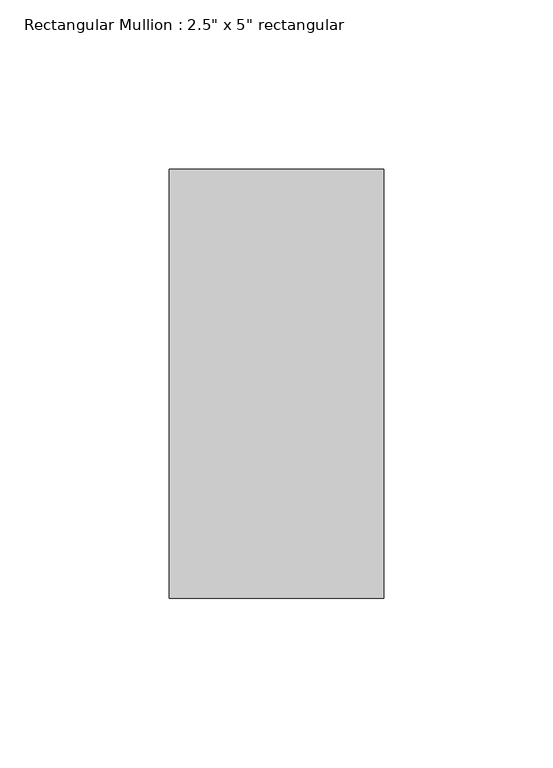
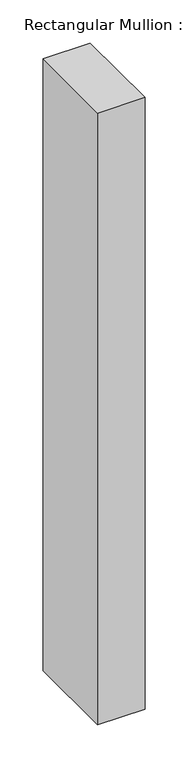
"""IFC4 building model written with IfcOpenShell, lengths in millimetres: member geometry."""

from ifc_helpers import new_model, si_unit, frame, origin, place, context, project, spatial, polyline, outline, extrude, source, transform, mapped, element, save


def member_bec57569(model_context):
    return source(origin(), model_context, "Body", "SweptSolid", [
        extrude(outline(polyline([(0.0, 63.5), (0.0, -63.5), (-63.5, -63.5), (-63.5, 63.5), (0.0, 63.5)])), frame((0.0, 0.0, -867.6657953), z_axis=(0.0, 0.0, 1.0), x_axis=(1.0, 0.0, 0.0)), (0.0, 0.0, 1.0), 867.6657953),
    ])


if __name__ == "__main__":
    model = new_model("IFC4")
    model_context = context("Model", 3, world=origin())
    ifc_project = project(units=[si_unit("LENGTHUNIT", "METRE", prefix="MILLI")], contexts=[model_context])
    site = spatial("IfcSite", under=ifc_project)
    building = spatial("IfcBuilding", under=site)
    placement = place(None, origin())
    member_shape = member_bec57569(model_context)
    element("IfcMember", 1, ObjectType="Rectangular Mullion : 2.5\" x 5\" rectangular", at=placement, inside=building, context=model_context, shape_type="MappedRepresentation", body=[
        mapped(member_shape, transform((0.0, 0.0, 0.0), x_axis=(1.0, 0.0, 0.0), y_axis=(0.0, 1.0, 0.0), z_axis=(0.0, 0.0, 1.0))),
    ])
    save(model, "model.ifc")

# Revit data of these elements
# Type "Rectangular Mullion : 2.5\" x 5\" rectangular"
#   built-in parameter 1007304 = 0.416667 (stored number, unit not read)
#   built-in parameter 1007301 = 0.104167 (stored number, unit not read)
#   built-in parameter 1007300 = 0.104167 (stored number, unit not read)
# Element 1 (IfcMember, "Rectangular Mullion : 2.5\" x 5\" rectangular")
#   Materials on its faces: "Aluminum"
# Materials
#   "Aluminum": class "Metal", colour RGB 247 247 247, transparency 0, Description = "Aluminum 6061", Cost = 0
